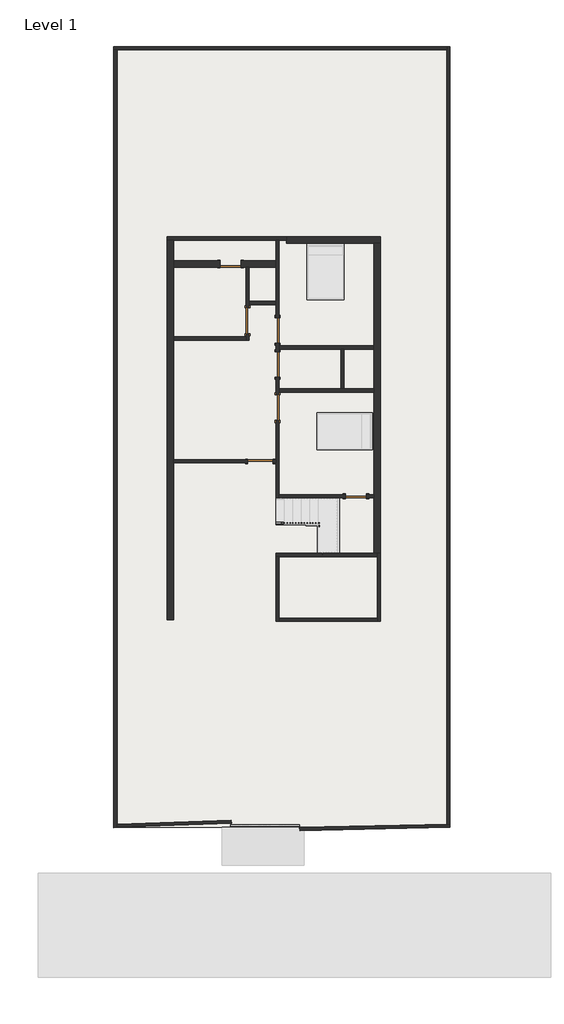
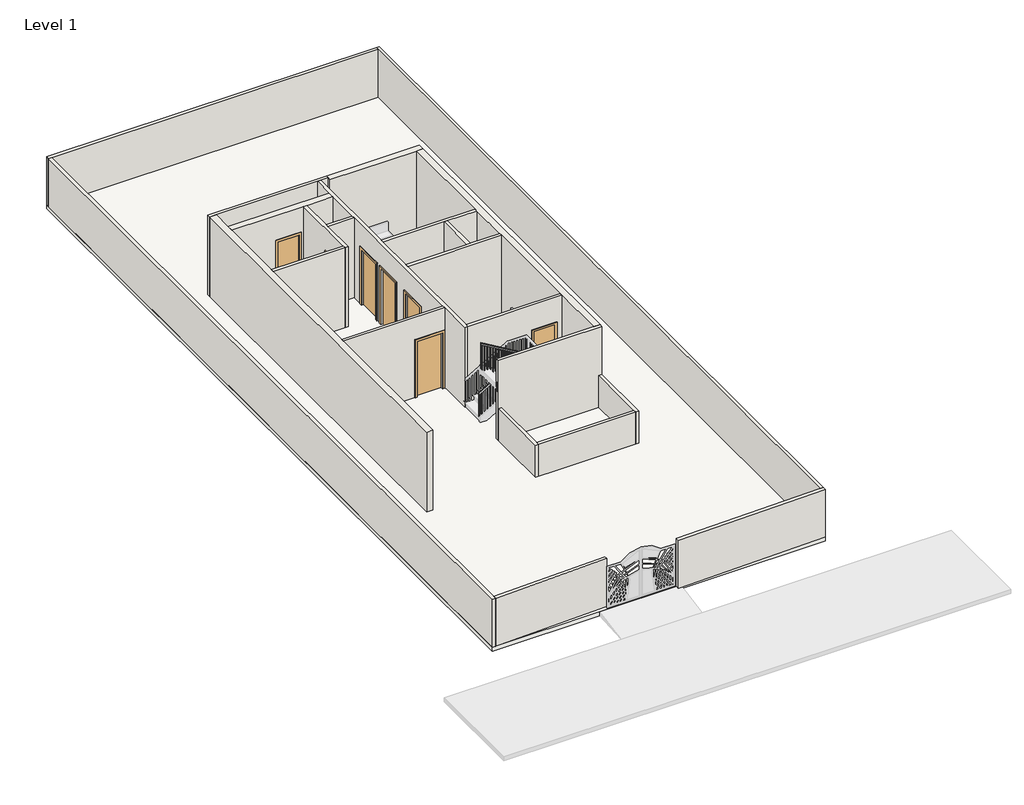
# One storey, part 1 of 2: 23 walls, 7 doors, 1 railing, 1 slab.
"""IFC4 building model written with IfcOpenShell, lengths in millimetres."""

from ifc_helpers import new_model, si_unit, frame, origin, origin_with_axes, place, context, project, spatial, polyline, outline, extrude, faceted_brep, transform, mapped, element, save
from components import door_85036156, door_d8f5dbb5, door_305aa2a5, door_e5f9f3c4

model = new_model("IFC4")

# Units and contexts
model_context = context("Model", 3, world=origin())
ifc_project = project(units=[si_unit("LENGTHUNIT", "METRE", prefix="MILLI")], contexts=[model_context])

# Site, building, storey
site = spatial("IfcSite", under=ifc_project)
building = spatial("IfcBuilding", under=site)
storey = spatial("IfcBuildingStorey", under=building, Name="Level 1", Elevation=0.0)

# Doors
placement = place(None, origin())
door_shape = door_85036156(model_context)
element("IfcDoor", 1, ObjectType="Single-Flush : 30\" x 80\"", at=placement, inside=storey, context=model_context, shape_type="MappedRepresentation", body=[
    mapped(door_shape, transform((-2798.2915084, 6430.9935985, 0.0), x_axis=(1.0, 0.0, 0.0), y_axis=(0.0, 1.0, 0.0), z_axis=(0.0, 0.0, 1.0))),
])
door_2_shape = door_d8f5dbb5(model_context)
element("IfcDoor", 2, ObjectType="Single-Flush : 30\" x 80\"", at=placement, inside=storey, context=model_context, shape_type="MappedRepresentation", body=[
    mapped(door_2_shape, transform((1678.4584916, -1855.7564015, 0.0), x_axis=(-1.0, 0.0, 0.0), y_axis=(0.0, -1.0, 0.0), z_axis=(0.0, 0.0, 1.0))),
])
door_3_shape = door_305aa2a5(model_context)
element("IfcDoor", 3, ObjectType="Single-Flush : 36\" x 84\"", at=placement, inside=storey, context=model_context, shape_type="MappedRepresentation", body=[
    mapped(door_3_shape, transform((-2188.6915084, 4405.3435985, 0.0), x_axis=(0.0, -1.0, 0.0), y_axis=(1.0, 0.0, 0.0), z_axis=(0.0, 0.0, 1.0))),
])
element("IfcDoor", 4, ObjectType="Single-Flush : 36\" x 84\"", at=placement, inside=storey, context=model_context, shape_type="MappedRepresentation", body=[
    mapped(door_3_shape, transform((-1121.8915084, 1306.5435985, 0.0), x_axis=(0.0, 1.0, 0.0), y_axis=(-1.0, 0.0, 0.0), z_axis=(0.0, 0.0, 1.0))),
])
door_4_shape = door_e5f9f3c4(model_context)
element("IfcDoor", 5, ObjectType="Single-Flush : 36\" x 84\"", at=placement, inside=storey, context=model_context, shape_type="MappedRepresentation", body=[
    mapped(door_4_shape, transform((-1121.8915084, 4062.4435985, 0.0), x_axis=(0.0, -1.0, 0.0), y_axis=(1.0, 0.0, 0.0), z_axis=(0.0, 0.0, 1.0))),
])
element("IfcDoor", 6, ObjectType="Single-Flush : 36\" x 84\"", at=placement, inside=storey, context=model_context, shape_type="MappedRepresentation", body=[
    mapped(door_4_shape, transform((-1121.8915084, 2843.2435985, 0.0), x_axis=(0.0, -1.0, 0.0), y_axis=(1.0, 0.0, 0.0), z_axis=(0.0, 0.0, 1.0))),
])
element("IfcDoor", 7, ObjectType="Single-Flush : 36\" x 84\"", at=placement, inside=storey, context=model_context, shape_type="MappedRepresentation", body=[
    mapped(door_4_shape, transform((-1731.4915084, -611.1564015, 0.0), x_axis=(1.0, 0.0, 0.0), y_axis=(0.0, 1.0, 0.0), z_axis=(0.0, 0.0, 1.0))),
])

# Railing
element("IfcRailing", 8, ObjectType="Handrail - Rectangular", at=placement, inside=storey, context=model_context, shape_type="SolidModel", body=[
    faceted_brep([(-1179.0415084, -2776.5064015, 1093.6941176), (-1179.0415084, -2776.5064015, 1034.7569051), (-1179.0415084, -2827.3064015, 1034.7569051), (-1179.0415084, -2827.3064015, 1093.6941176), (268.7584916, -2776.5064015, 1945.3411765), (319.5584916, -2776.5064015, 1916.2863169), (319.5584916, -2827.3064015, 1916.2863169), (268.7584916, -2827.3064015, 1945.3411765), (268.7584916, -2776.5064015, 1990.1647059), (319.5584916, -2776.5064015, 1939.3647059), (319.5584916, -2827.3064015, 1939.3647059), (268.7584916, -2827.3064015, 1990.1647059), (395.7584916, -2776.5064015, 1990.1647059), (395.7584916, -2776.5064015, 1939.3647059), (344.9584916, -2827.3064015, 1939.3647059), (344.9584916, -2827.3064015, 1990.1647059), (395.7584916, -2903.5064015, 1990.1647059), (395.7584916, -2903.5064015, 1939.3647059), (344.9584916, -2903.5064015, 1939.3647059), (344.9584916, -2903.5064015, 1990.1647059), (395.7584916, -2928.9064015, 1990.1647059), (344.9584916, -2928.9064015, 1990.1647059), (344.9584916, -2928.9064015, 1939.3647059), (395.7584916, -2928.9064015, 1939.3647059)], [[[0, 1, 2, 3]], [[1, 0, 4, 5]], [[2, 1, 5, 6]], [[3, 2, 6, 7]], [[0, 3, 7, 4]], [[5, 4, 8, 9]], [[6, 5, 9, 10]], [[7, 6, 10, 11]], [[4, 7, 11, 8]], [[9, 8, 12, 13]], [[10, 9, 13, 14]], [[11, 10, 14, 15]], [[8, 11, 15, 12]], [[13, 12, 16, 17]], [[14, 13, 17, 18]], [[15, 14, 18, 19]], [[12, 15, 19, 16]], [[20, 21, 22, 23]], [[17, 16, 20, 23]], [[18, 17, 23, 22]], [[19, 18, 22, 21]], [[16, 19, 21, 20]]]),
    faceted_brep([(395.7584916, -2903.5064015, 1990.1647059), (395.7584916, -2954.3064015, 1939.3647059), (344.9584916, -2954.3064015, 1939.3647059), (344.9584916, -2903.5064015, 1990.1647059), (395.7584916, -2903.5064015, 2139.5764706), (344.9584916, -2903.5064015, 2110.521611), (344.9584916, -2954.3064015, 2110.521611), (395.7584916, -2954.3064015, 2139.5764706)], [[[0, 1, 2, 3]], [[4, 5, 6, 7]], [[1, 0, 4, 7]], [[2, 1, 7, 6]], [[3, 2, 6, 5]], [[0, 3, 5, 4]]]),
    faceted_brep([(395.7584916, -2954.3064015, 2139.5764706), (344.9584916, -2954.3064015, 2110.521611), (344.9584916, -2903.5064015, 2110.521611), (395.7584916, -2903.5064015, 2139.5764706), (-1179.0415084, -2954.3064015, 3065.9294118), (-1179.0415084, -2903.5064015, 3065.9294118), (-1179.0415084, -2903.5064015, 3006.9921993), (-1179.0415084, -2954.3064015, 3006.9921993)], [[[0, 1, 2, 3]], [[4, 5, 6, 7]], [[1, 0, 4, 7]], [[2, 1, 7, 6]], [[3, 2, 6, 5]], [[0, 3, 5, 4]]]),
    extrude(outline(polyline([(2986.4480816, -1144.1165084), (2997.653964, -1163.1665084), (1972.2352941, -1163.1665084), (1972.2352941, -1144.1165084), (2986.4480816, -1144.1165084)])), frame((0.0, -2938.4314015, 0.0), z_axis=(0.0, 1.0, 0.0), x_axis=(0.0, 0.0, 1.0)), (0.0, 0.0, 1.0), 19.05),
    extrude(outline(polyline([(2926.6833757, -1042.5165084), (2937.8892581, -1061.5665084), (1972.2352941, -1061.5665084), (1972.2352941, -1042.5165084), (2926.6833757, -1042.5165084)])), frame((0.0, -2938.4314015, 0.0), z_axis=(0.0, 1.0, 0.0), x_axis=(0.0, 0.0, 1.0)), (0.0, 0.0, 1.0), 19.05),
    extrude(outline(polyline([(2866.9186699, -940.9165084), (2878.1245522, -959.9665084), (1972.2352941, -959.9665084), (1972.2352941, -940.9165084), (2866.9186699, -940.9165084)])), frame((0.0, -2938.4314015, 0.0), z_axis=(0.0, 1.0, 0.0), x_axis=(0.0, 0.0, 1.0)), (0.0, 0.0, 1.0), 19.05),
    extrude(outline(polyline([(2807.153964, -839.3165084), (2818.3598463, -858.3665084), (1792.9411765, -858.3665084), (1792.9411765, -839.3165084), (2807.153964, -839.3165084)])), frame((0.0, -2938.4314015, 0.0), z_axis=(0.0, 1.0, 0.0), x_axis=(0.0, 0.0, 1.0)), (0.0, 0.0, 1.0), 19.05),
    extrude(outline(polyline([(2747.3892581, -737.7165084), (2758.5951404, -756.7665084), (1792.9411765, -756.7665084), (1792.9411765, -737.7165084), (2747.3892581, -737.7165084)])), frame((0.0, -2938.4314015, 0.0), z_axis=(0.0, 1.0, 0.0), x_axis=(0.0, 0.0, 1.0)), (0.0, 0.0, 1.0), 19.05),
    extrude(outline(polyline([(2687.6245522, -636.1165084), (2698.8304346, -655.1665084), (1792.9411765, -655.1665084), (1792.9411765, -636.1165084), (2687.6245522, -636.1165084)])), frame((0.0, -2938.4314015, 0.0), z_axis=(0.0, 1.0, 0.0), x_axis=(0.0, 0.0, 1.0)), (0.0, 0.0, 1.0), 19.05),
    extrude(outline(polyline([(2627.8598463, -534.5165084), (2639.0657287, -553.5665084), (1613.6470588, -553.5665084), (1613.6470588, -534.5165084), (2627.8598463, -534.5165084)])), frame((0.0, -2938.4314015, 0.0), z_axis=(0.0, 1.0, 0.0), x_axis=(0.0, 0.0, 1.0)), (0.0, 0.0, 1.0), 19.05),
    extrude(outline(polyline([(2568.0951404, -432.9165084), (2579.3010228, -451.9665084), (1613.6470588, -451.9665084), (1613.6470588, -432.9165084), (2568.0951404, -432.9165084)])), frame((0.0, -2938.4314015, 0.0), z_axis=(0.0, 1.0, 0.0), x_axis=(0.0, 0.0, 1.0)), (0.0, 0.0, 1.0), 19.05),
    extrude(outline(polyline([(2508.3304346, -331.3165084), (2519.5363169, -350.3665084), (1613.6470588, -350.3665084), (1613.6470588, -331.3165084), (2508.3304346, -331.3165084)])), frame((0.0, -2938.4314015, 0.0), z_axis=(0.0, 1.0, 0.0), x_axis=(0.0, 0.0, 1.0)), (0.0, 0.0, 1.0), 19.05),
    extrude(outline(polyline([(2448.5657287, -229.7165084), (2459.771611, -248.7665084), (1434.3529412, -248.7665084), (1434.3529412, -229.7165084), (2448.5657287, -229.7165084)])), frame((0.0, -2938.4314015, 0.0), z_axis=(0.0, 1.0, 0.0), x_axis=(0.0, 0.0, 1.0)), (0.0, 0.0, 1.0), 19.05),
    extrude(outline(polyline([(2388.8010228, -128.1165084), (2400.0069051, -147.1665084), (1434.3529412, -147.1665084), (1434.3529412, -128.1165084), (2388.8010228, -128.1165084)])), frame((0.0, -2938.4314015, 0.0), z_axis=(0.0, 1.0, 0.0), x_axis=(0.0, 0.0, 1.0)), (0.0, 0.0, 1.0), 19.05),
    extrude(outline(polyline([(2329.0363169, -26.5165084), (2340.2421993, -45.5665084), (1434.3529412, -45.5665084), (1434.3529412, -26.5165084), (2329.0363169, -26.5165084)])), frame((0.0, -2938.4314015, 0.0), z_axis=(0.0, 1.0, 0.0), x_axis=(0.0, 0.0, 1.0)), (0.0, 0.0, 1.0), 19.05),
    extrude(outline(polyline([(2269.271611, 75.0834916), (2280.4774934, 56.0334916), (1255.0588235, 56.0334916), (1255.0588235, 75.0834916), (2269.271611, 75.0834916)])), frame((0.0, -2938.4314015, 0.0), z_axis=(0.0, 1.0, 0.0), x_axis=(0.0, 0.0, 1.0)), (0.0, 0.0, 1.0), 19.05),
    extrude(outline(polyline([(2209.5069051, 176.6834916), (2220.7127875, 157.6334916), (1255.0588235, 157.6334916), (1255.0588235, 176.6834916), (2209.5069051, 176.6834916)])), frame((0.0, -2938.4314015, 0.0), z_axis=(0.0, 1.0, 0.0), x_axis=(0.0, 0.0, 1.0)), (0.0, 0.0, 1.0), 19.05),
    extrude(outline(polyline([(2149.7421993, 278.2834916), (2160.9480816, 259.2334916), (1255.0588235, 259.2334916), (1255.0588235, 278.2834916), (2149.7421993, 278.2834916)])), frame((0.0, -2938.4314015, 0.0), z_axis=(0.0, 1.0, 0.0), x_axis=(0.0, 0.0, 1.0)), (0.0, 0.0, 1.0), 19.05),
    extrude(outline(polyline([(360.8334916, -2893.9814015), (379.8834916, -2893.9814015), (379.8834916, -2913.0314015), (360.8334916, -2913.0314015), (360.8334916, -2893.9814015)])), frame((0.0, 0.0, 1075.7647059), z_axis=(0.0, 0.0, 1.0), x_axis=(1.0, 0.0, 0.0)), (0.0, 0.0, 1.0), 863.6),
    extrude(outline(polyline([(335.4334916, -2811.4314015), (335.4334916, -2792.3814015), (354.4834916, -2792.3814015), (354.4834916, -2811.4314015), (335.4334916, -2811.4314015)])), frame((0.0, 0.0, 1075.7647059), z_axis=(0.0, 0.0, 1.0), x_axis=(1.0, 0.0, 0.0)), (0.0, 0.0, 1.0), 863.6),
    extrude(outline(polyline([(1877.0657287, 252.8834916), (1865.8598463, 233.8334916), (896.4705882, 233.8334916), (896.4705882, 252.8834916), (1877.0657287, 252.8834916)])), frame((0.0, -2811.4314015, 0.0), z_axis=(0.0, 1.0, 0.0), x_axis=(0.0, 0.0, 1.0)), (0.0, 0.0, 1.0), 19.05),
    extrude(outline(polyline([(1817.3010228, 151.2834916), (1806.0951404, 132.2334916), (896.4705882, 132.2334916), (896.4705882, 151.2834916), (1817.3010228, 151.2834916)])), frame((0.0, -2811.4314015, 0.0), z_axis=(0.0, 1.0, 0.0), x_axis=(0.0, 0.0, 1.0)), (0.0, 0.0, 1.0), 19.05),
    extrude(outline(polyline([(1757.5363169, 49.6834916), (1746.3304346, 30.6334916), (896.4705882, 30.6334916), (896.4705882, 49.6834916), (1757.5363169, 49.6834916)])), frame((0.0, -2811.4314015, 0.0), z_axis=(0.0, 1.0, 0.0), x_axis=(0.0, 0.0, 1.0)), (0.0, 0.0, 1.0), 19.05),
    extrude(outline(polyline([(1697.771611, -51.9165084), (1686.5657287, -70.9665084), (717.1764706, -70.9665084), (717.1764706, -51.9165084), (1697.771611, -51.9165084)])), frame((0.0, -2811.4314015, 0.0), z_axis=(0.0, 1.0, 0.0), x_axis=(0.0, 0.0, 1.0)), (0.0, 0.0, 1.0), 19.05),
    extrude(outline(polyline([(1638.0069051, -153.5165084), (1626.8010228, -172.5665084), (717.1764706, -172.5665084), (717.1764706, -153.5165084), (1638.0069051, -153.5165084)])), frame((0.0, -2811.4314015, 0.0), z_axis=(0.0, 1.0, 0.0), x_axis=(0.0, 0.0, 1.0)), (0.0, 0.0, 1.0), 19.05),
    extrude(outline(polyline([(1578.2421993, -255.1165084), (1567.0363169, -274.1665084), (717.1764706, -274.1665084), (717.1764706, -255.1165084), (1578.2421993, -255.1165084)])), frame((0.0, -2811.4314015, 0.0), z_axis=(0.0, 1.0, 0.0), x_axis=(0.0, 0.0, 1.0)), (0.0, 0.0, 1.0), 19.05),
    extrude(outline(polyline([(1518.4774934, -356.7165084), (1507.271611, -375.7665084), (537.8823529, -375.7665084), (537.8823529, -356.7165084), (1518.4774934, -356.7165084)])), frame((0.0, -2811.4314015, 0.0), z_axis=(0.0, 1.0, 0.0), x_axis=(0.0, 0.0, 1.0)), (0.0, 0.0, 1.0), 19.05),
    extrude(outline(polyline([(1458.7127875, -458.3165084), (1447.5069051, -477.3665084), (537.8823529, -477.3665084), (537.8823529, -458.3165084), (1458.7127875, -458.3165084)])), frame((0.0, -2811.4314015, 0.0), z_axis=(0.0, 1.0, 0.0), x_axis=(0.0, 0.0, 1.0)), (0.0, 0.0, 1.0), 19.05),
    extrude(outline(polyline([(1398.9480816, -559.9165084), (1387.7421993, -578.9665084), (537.8823529, -578.9665084), (537.8823529, -559.9165084), (1398.9480816, -559.9165084)])), frame((0.0, -2811.4314015, 0.0), z_axis=(0.0, 1.0, 0.0), x_axis=(0.0, 0.0, 1.0)), (0.0, 0.0, 1.0), 19.05),
    extrude(outline(polyline([(1339.1833757, -661.5165084), (1327.9774934, -680.5665084), (358.5882353, -680.5665084), (358.5882353, -661.5165084), (1339.1833757, -661.5165084)])), frame((0.0, -2811.4314015, 0.0), z_axis=(0.0, 1.0, 0.0), x_axis=(0.0, 0.0, 1.0)), (0.0, 0.0, 1.0), 19.05),
    extrude(outline(polyline([(1279.4186699, -763.1165084), (1268.2127875, -782.1665084), (358.5882353, -782.1665084), (358.5882353, -763.1165084), (1279.4186699, -763.1165084)])), frame((0.0, -2811.4314015, 0.0), z_axis=(0.0, 1.0, 0.0), x_axis=(0.0, 0.0, 1.0)), (0.0, 0.0, 1.0), 19.05),
    extrude(outline(polyline([(1219.653964, -864.7165084), (1208.4480816, -883.7665084), (358.5882353, -883.7665084), (358.5882353, -864.7165084), (1219.653964, -864.7165084)])), frame((0.0, -2811.4314015, 0.0), z_axis=(0.0, 1.0, 0.0), x_axis=(0.0, 0.0, 1.0)), (0.0, 0.0, 1.0), 19.05),
    extrude(outline(polyline([(1159.8892581, -966.3165084), (1148.6833757, -985.3665084), (179.2941176, -985.3665084), (179.2941176, -966.3165084), (1159.8892581, -966.3165084)])), frame((0.0, -2811.4314015, 0.0), z_axis=(0.0, 1.0, 0.0), x_axis=(0.0, 0.0, 1.0)), (0.0, 0.0, 1.0), 19.05),
    extrude(outline(polyline([(1100.1245522, -1067.9165084), (1088.9186699, -1086.9665084), (179.2941176, -1086.9665084), (179.2941176, -1067.9165084), (1100.1245522, -1067.9165084)])), frame((0.0, -2811.4314015, 0.0), z_axis=(0.0, 1.0, 0.0), x_axis=(0.0, 0.0, 1.0)), (0.0, 0.0, 1.0), 19.05),
    extrude(outline(polyline([(360.8334916, -2919.3814015), (379.8834916, -2919.3814015), (379.8834916, -2938.4314015), (360.8334916, -2938.4314015), (360.8334916, -2919.3814015)])), frame((0.0, 0.0, 1075.7647059), z_axis=(0.0, 0.0, 1.0), x_axis=(1.0, 0.0, 0.0)), (0.0, 0.0, 1.0), 863.6),
    extrude(outline(polyline([(360.8334916, -2811.4314015), (360.8334916, -2792.3814015), (379.8834916, -2792.3814015), (379.8834916, -2811.4314015), (360.8334916, -2811.4314015)])), frame((0.0, 0.0, 1075.7647059), z_axis=(0.0, 0.0, 1.0), x_axis=(1.0, 0.0, 0.0)), (0.0, 0.0, 1.0), 863.6),
    extrude(outline(polyline([(2995.7863169, -1159.9915084), (3006.9921993, -1179.0415084), (1972.2352941, -1179.0415084), (1972.2352941, -1159.9915084), (2995.7863169, -1159.9915084)])), frame((0.0, -2938.4314015, 0.0), z_axis=(0.0, 1.0, 0.0), x_axis=(0.0, 0.0, 1.0)), (0.0, 0.0, 1.0), 19.05),
    extrude(outline(polyline([(1045.9627875, -1159.9915084), (1034.7569051, -1179.0415084), (179.2941176, -1179.0415084), (179.2941176, -1159.9915084), (1045.9627875, -1159.9915084)])), frame((0.0, -2811.4314015, 0.0), z_axis=(0.0, 1.0, 0.0), x_axis=(0.0, 0.0, 1.0)), (0.0, 0.0, 1.0), 19.05),
])

# Slab
element("IfcSlab", 9, ObjectType="Generic - 12\"", at=placement, inside=storey, context=model_context, shape_type="SweptSolid", body=[
    extrude(outline(polyline([(5035.3021219, 14183.4869538), (5035.3021219, -13665.8789629), (-6966.1978781, -13665.8789629), (-6966.1978781, 14183.4869538), (5035.3021219, 14183.4869538)])), frame((0.0, 0.0, -152.4), z_axis=(0.0, 0.0, 1.0), x_axis=(1.0, 0.0, 0.0)), (0.0, 0.0, 1.0), 152.4),
])

# Walls
element("IfcWall", 10, ObjectType="WALL 9\"", at=placement, inside=storey, context=model_context, shape_type="Brep", body=[
    faceted_brep([(-798.0415084, 7167.5935985, 0.0), (2326.1584916, 7167.5935985, 0.0), (2554.7584916, 7167.5935985, 0.0), (2554.7584916, 7167.5935985, 3048.0), (2326.1584916, 7167.5935985, 3048.0), (-798.0415084, 7167.5935985, 3048.0), (-798.0415084, 7396.1935985, 0.0), (-798.0415084, 7396.1935985, 3048.0), (2554.7584916, 7396.1935985, 3048.0), (2554.7584916, 7396.1935985, 0.0), (-798.0415084, 7281.8935985, 0.0), (-798.0415084, 7281.8935985, 3048.0)], [[[0, 1, 2, 3, 4, 5]], [[6, 7, 8, 9]], [[2, 1, 0, 10, 6, 9]], [[0, 5, 11, 7, 6, 10]], [[3, 2, 9, 8]], [[5, 4, 3, 8, 7, 11]]]),
])
element("IfcWall", 11, ObjectType="WALL 9\"", at=placement, inside=storey, context=model_context, shape_type="Brep", body=[
    faceted_brep([(2326.1584916, 7167.5935985, 0.0), (2326.1584916, 3509.9935985, 0.0), (2326.1584916, 3395.6935985, 0.0), (2326.1584916, 1973.2935985, 0.0), (2326.1584916, 1858.9935985, 0.0), (2326.1584916, -1798.6064015, 0.0), (2326.1584916, -1912.9064015, 0.0), (2326.1584916, -3894.1064015, 0.0), (2326.1584916, -3894.1064015, 3048.0), (2326.1584916, -1912.9064015, 3048.0), (2326.1584916, -1798.6064015, 3048.0), (2326.1584916, 1858.9935985, 3048.0), (2326.1584916, 1973.2935985, 3048.0), (2326.1584916, 3395.6935985, 3048.0), (2326.1584916, 3509.9935985, 3048.0), (2326.1584916, 7167.5935985, 3048.0), (2554.7584916, 7167.5935985, 0.0), (2554.7584916, 7167.5935985, 3048.0), (2554.7584916, -3894.1064015, 3048.0), (2554.7584916, -3894.1064015, 1219.2), (2554.7584916, -3894.1064015, 0.0), (2440.4584916, -3894.1064015, 0.0)], [[[0, 1, 2, 3, 4, 5, 6, 7, 8, 9, 10, 11, 12, 13, 14, 15]], [[16, 17, 18, 19, 20]], [[7, 6, 5, 4, 3, 2, 1, 0, 16, 20, 21]], [[0, 15, 17, 16]], [[8, 7, 21, 20, 19, 18]], [[15, 14, 13, 12, 11, 10, 9, 8, 18, 17]]]),
])
element("IfcWall", 12, ObjectType="WALL 9\"", at=placement, inside=storey, context=model_context, shape_type="Brep", body=[
    faceted_brep([(-5065.2415084, 7281.8935985, 0.0), (-5065.2415084, -6262.6564015, 0.0), (-5065.2415084, -6262.6564015, 3048.0), (-5065.2415084, 7281.8935985, 3048.0), (-4836.6415084, 7281.8935985, 0.0), (-4836.6415084, 7281.8935985, 3048.0), (-4836.6415084, 6545.2935985, 3048.0), (-4836.6415084, 6316.6935985, 3048.0), (-4836.6415084, 3827.4935985, 3048.0), (-4836.6415084, 3713.1935985, 3048.0), (-4836.6415084, -554.0064015, 3048.0), (-4836.6415084, -668.3064015, 3048.0), (-4836.6415084, -6262.6564015, 3048.0), (-4836.6415084, -6262.6564015, 0.0), (-4836.6415084, -668.3064015, 0.0), (-4836.6415084, -554.0064015, 0.0), (-4836.6415084, 3713.1935985, 0.0), (-4836.6415084, 3827.4935985, 0.0), (-4836.6415084, 6316.6935985, 0.0), (-4836.6415084, 6545.2935985, 0.0)], [[[0, 1, 2, 3]], [[4, 5, 6, 7, 8, 9, 10, 11, 12, 13, 14, 15, 16, 17, 18, 19]], [[1, 0, 4, 19, 18, 17, 16, 15, 14, 13]], [[2, 1, 13, 12]], [[0, 3, 5, 4]], [[3, 2, 12, 11, 10, 9, 8, 7, 6, 5]]]),
])
element("IfcWall", 13, ObjectType="WALL 9\"", at=placement, inside=storey, context=model_context, shape_type="Brep", body=[
    faceted_brep([(-2417.2915084, 6316.6935985, 2032.0), (-2417.2915084, 6316.6935985, 0.0), (-2245.8415084, 6316.6935985, 0.0), (-2131.5415084, 6316.6935985, 0.0), (-1179.0415084, 6316.6935985, 0.0), (-1179.0415084, 6316.6935985, 3048.0), (-2131.5415084, 6316.6935985, 3048.0), (-2245.8415084, 6316.6935985, 3048.0), (-4836.6415084, 6316.6935985, 3048.0), (-4836.6415084, 6316.6935985, 0.0), (-3179.2915084, 6316.6935985, 0.0), (-3179.2915084, 6316.6935985, 2032.0), (-1179.0415084, 6545.2935985, 0.0), (-2417.2915084, 6545.2935985, 0.0), (-2417.2915084, 6545.2935985, 2032.0), (-3179.2915084, 6545.2935985, 2032.0), (-3179.2915084, 6545.2935985, 0.0), (-4836.6415084, 6545.2935985, 0.0), (-4836.6415084, 6545.2935985, 3048.0), (-1179.0415084, 6545.2935985, 3048.0)], [[[0, 1, 2, 3, 4, 5, 6, 7, 8, 9, 10, 11]], [[12, 13, 14, 15, 16, 17, 18, 19]], [[10, 9, 17, 16]], [[4, 3, 2, 1, 13, 12]], [[9, 8, 18, 17]], [[5, 4, 12, 19]], [[14, 13, 1, 0]], [[15, 14, 0, 11]], [[16, 15, 11, 10]], [[8, 7, 6, 5, 19, 18]]]),
])
element("IfcWall", 14, ObjectType="WALL4.5\"", at=placement, inside=storey, context=model_context, shape_type="Brep", body=[
    faceted_brep([(-5065.2415084, 7281.8935985, 0.0), (-4836.6415084, 7281.8935985, 0.0), (-1179.0415084, 7281.8935985, 0.0), (-1064.7415084, 7281.8935985, 0.0), (-798.0415084, 7281.8935985, 0.0), (-798.0415084, 7281.8935985, 3048.0), (-1064.7415084, 7281.8935985, 3048.0), (-1179.0415084, 7281.8935985, 3048.0), (-4836.6415084, 7281.8935985, 3048.0), (-5065.2415084, 7281.8935985, 3048.0), (-5065.2415084, 7396.1935985, 0.0), (-5065.2415084, 7396.1935985, 3048.0), (-798.0415084, 7396.1935985, 3048.0), (-798.0415084, 7396.1935985, 0.0)], [[[0, 1, 2, 3, 4, 5, 6, 7, 8, 9]], [[10, 11, 12, 13]], [[4, 3, 2, 1, 0, 10, 13]], [[5, 4, 13, 12]], [[0, 9, 11, 10]], [[9, 8, 7, 6, 5, 12, 11]]]),
])
element("IfcWall", 15, ObjectType="WALL4.5\"", at=placement, inside=storey, context=model_context, shape_type="Brep", body=[
    faceted_brep([(2554.7584916, -6319.8064015, 0.0), (2554.7584916, -3894.1064015, 0.0), (2554.7584916, -3894.1064015, 1219.2), (2554.7584916, -4008.4064015, 1219.2), (2554.7584916, -6319.8064015, 1219.2), (2440.4584916, -6319.8064015, 0.0), (2440.4584916, -6319.8064015, 1219.2), (2440.4584916, -6205.5064015, 1219.2), (2440.4584916, -4008.4064015, 1219.2), (2440.4584916, -3894.1064015, 1219.2), (2440.4584916, -3894.1064015, 0.0), (2440.4584916, -4008.4064015, 0.0), (2440.4584916, -6205.5064015, 0.0)], [[[0, 1, 2, 3, 4]], [[5, 6, 7, 8, 9, 10, 11, 12]], [[1, 0, 5, 12, 11, 10]], [[4, 3, 2, 9, 8, 7, 6]], [[2, 1, 10, 9]], [[0, 4, 6, 5]]]),
])
element("IfcWall", 16, ObjectType="WALL4.5\"", at=placement, inside=storey, context=model_context, shape_type="Brep", body=[
    faceted_brep([(2440.4584916, -3894.1064015, 0.0), (2326.1584916, -3894.1064015, 0.0), (-1179.0415084, -3894.1064015, 0.0), (-1179.0415084, -3894.1064015, 3048.0), (2326.1584916, -3894.1064015, 3048.0), (2554.7584916, -3894.1064015, 3048.0), (2554.7584916, -3894.1064015, 1219.2), (2440.4584916, -3894.1064015, 1219.2), (2440.4584916, -4008.4064015, 0.0), (2440.4584916, -4008.4064015, 1219.2), (2554.7584916, -4008.4064015, 1219.2), (2554.7584916, -4008.4064015, 3048.0), (-1179.0415084, -4008.4064015, 3048.0), (-1179.0415084, -4008.4064015, 1219.2), (-1179.0415084, -4008.4064015, 0.0), (-1064.7415084, -4008.4064015, 0.0)], [[[0, 1, 2, 3, 4, 5, 6, 7]], [[8, 9, 10, 11, 12, 13, 14, 15]], [[2, 1, 0, 8, 15, 14]], [[3, 2, 14, 13, 12]], [[6, 10, 9, 7]], [[0, 7, 9, 8]], [[6, 5, 11, 10]], [[5, 4, 3, 12, 11]]]),
])
element("IfcWall", 17, ObjectType="WALL4.5\"", at=placement, inside=storey, context=model_context, shape_type="Brep", body=[
    faceted_brep([(-2245.8415084, 3948.1435985, 2133.6), (-2245.8415084, 3948.1435985, 0.0), (-2245.8415084, 3827.4935985, 0.0), (-2245.8415084, 3713.1935985, 0.0), (-2245.8415084, 3713.1935985, 3048.0), (-2245.8415084, 3827.4935985, 3048.0), (-2245.8415084, 6316.6935985, 3048.0), (-2245.8415084, 6316.6935985, 0.0), (-2245.8415084, 4862.5435985, 0.0), (-2245.8415084, 4862.5435985, 2133.6), (-2131.5415084, 3713.1935985, 0.0), (-2131.5415084, 3948.1435985, 0.0), (-2131.5415084, 3948.1435985, 2133.6), (-2131.5415084, 4862.5435985, 2133.6), (-2131.5415084, 4862.5435985, 0.0), (-2131.5415084, 4983.1935985, 0.0), (-2131.5415084, 5097.4935985, 0.0), (-2131.5415084, 6316.6935985, 0.0), (-2131.5415084, 6316.6935985, 3048.0), (-2131.5415084, 5097.4935985, 3048.0), (-2131.5415084, 4983.1935985, 3048.0), (-2131.5415084, 3713.1935985, 3048.0)], [[[0, 1, 2, 3, 4, 5, 6, 7, 8, 9]], [[10, 11, 12, 13, 14, 15, 16, 17, 18, 19, 20, 21]], [[8, 7, 17, 16, 15, 14]], [[3, 2, 1, 11, 10]], [[7, 6, 18, 17]], [[4, 3, 10, 21]], [[12, 11, 1, 0]], [[13, 12, 0, 9]], [[14, 13, 9, 8]], [[6, 5, 4, 21, 20, 19, 18]]]),
])
element("IfcWall", 18, ObjectType="WALL4.5\"", at=placement, inside=storey, context=model_context, shape_type="SweptSolid", body=[
    extrude(outline(polyline([(-2245.8415084, 3713.1935985), (-4836.6415084, 3713.1935985), (-4836.6415084, 3827.4935985), (-2245.8415084, 3827.4935985), (-2245.8415084, 3713.1935985)])), origin_with_axes(), (0.0, 0.0, 1.0), 3048.0),
])
element("IfcWall", 19, ObjectType="WALL4.5\"", at=placement, inside=storey, context=model_context, shape_type="SweptSolid", body=[
    extrude(outline(polyline([(-1179.0415084, 4983.1935985), (-2131.5415084, 4983.1935985), (-2131.5415084, 5097.4935985), (-1179.0415084, 5097.4935985), (-1179.0415084, 4983.1935985)])), origin_with_axes(), (0.0, 0.0, 1.0), 3048.0),
])
element("IfcWall", 20, ObjectType="WALL4.5\"", at=placement, inside=storey, context=model_context, shape_type="Brep", body=[
    faceted_brep([(-1179.0415084, 2386.0435985, 0.0), (-1179.0415084, 1763.7435985, 0.0), (-1179.0415084, 1763.7435985, 2133.6), (-1179.0415084, 849.3435985, 2133.6), (-1179.0415084, 849.3435985, 0.0), (-1179.0415084, -554.0064015, 0.0), (-1179.0415084, -668.3064015, 0.0), (-1179.0415084, -1912.9064015, 0.0), (-1179.0415084, -1912.9064015, 3048.0), (-1179.0415084, -668.3064015, 3048.0), (-1179.0415084, -554.0064015, 3048.0), (-1179.0415084, 4983.1935985, 3048.0), (-1179.0415084, 5097.4935985, 3048.0), (-1179.0415084, 6316.6935985, 3048.0), (-1179.0415084, 6545.2935985, 3048.0), (-1179.0415084, 7281.8935985, 3048.0), (-1179.0415084, 7281.8935985, 0.0), (-1179.0415084, 6545.2935985, 0.0), (-1179.0415084, 6316.6935985, 0.0), (-1179.0415084, 5097.4935985, 0.0), (-1179.0415084, 4983.1935985, 0.0), (-1179.0415084, 4519.6435985, 0.0), (-1179.0415084, 4519.6435985, 2133.6), (-1179.0415084, 3605.2435985, 2133.6), (-1179.0415084, 3605.2435985, 0.0), (-1179.0415084, 3300.4435985, 0.0), (-1179.0415084, 3300.4435985, 2133.6), (-1179.0415084, 2386.0435985, 2133.6), (-1064.7415084, 1763.7435985, 2133.6), (-1064.7415084, 1763.7435985, 0.0), (-1064.7415084, 1858.9935985, 0.0), (-1064.7415084, 1973.2935985, 0.0), (-1064.7415084, 2386.0435985, 0.0), (-1064.7415084, 2386.0435985, 2133.6), (-1064.7415084, 3300.4435985, 2133.6), (-1064.7415084, 3300.4435985, 0.0), (-1064.7415084, 3395.6935985, 0.0), (-1064.7415084, 3509.9935985, 0.0), (-1064.7415084, 3605.2435985, 0.0), (-1064.7415084, 3605.2435985, 2133.6), (-1064.7415084, 4519.6435985, 2133.6), (-1064.7415084, 4519.6435985, 0.0), (-1064.7415084, 7281.8935985, 0.0), (-1064.7415084, 7281.8935985, 3048.0), (-1064.7415084, 3509.9935985, 3048.0), (-1064.7415084, 3395.6935985, 3048.0), (-1064.7415084, 1973.2935985, 3048.0), (-1064.7415084, 1858.9935985, 3048.0), (-1064.7415084, -1798.6064015, 3048.0), (-1064.7415084, -1912.9064015, 3048.0), (-1064.7415084, -1912.9064015, 0.0), (-1064.7415084, -1798.6064015, 0.0), (-1064.7415084, 849.3435985, 0.0), (-1064.7415084, 849.3435985, 2133.6)], [[[0, 1, 2, 3, 4, 5, 6, 7, 8, 9, 10, 11, 12, 13, 14, 15, 16, 17, 18, 19, 20, 21, 22, 23, 24, 25, 26, 27]], [[28, 29, 30, 31, 32, 33, 34, 35, 36, 37, 38, 39, 40, 41, 42, 43, 44, 45, 46, 47, 48, 49, 50, 51, 52, 53]], [[21, 20, 19, 18, 17, 16, 42, 41]], [[25, 24, 38, 37, 36, 35]], [[52, 51, 50, 7, 6, 5, 4]], [[32, 31, 30, 29, 1, 0]], [[16, 15, 43, 42]], [[8, 7, 50, 49]], [[39, 38, 24, 23]], [[40, 39, 23, 22]], [[41, 40, 22, 21]], [[33, 32, 0, 27]], [[34, 33, 27, 26]], [[35, 34, 26, 25]], [[2, 1, 29, 28]], [[3, 2, 28, 53]], [[4, 3, 53, 52]], [[15, 14, 13, 12, 11, 10, 9, 8, 49, 48, 47, 46, 45, 44, 43]]]),
])
element("IfcWall", 21, ObjectType="WALL4.5\"", at=placement, inside=storey, context=model_context, shape_type="SweptSolid", body=[
    extrude(outline(polyline([(0.0, -1064.7415084), (0.0, 1297.4584916), (2032.0, 1297.4584916), (2032.0, 2059.4584916), (0.0, 2059.4584916), (0.0, 2326.1584916), (3048.0, 2326.1584916), (3048.0, -1064.7415084), (0.0, -1064.7415084)])), frame((0.0, -1912.9064015, 0.0), z_axis=(0.0, 1.0, 0.0), x_axis=(0.0, 0.0, 1.0)), (0.0, 0.0, 1.0), 114.3),
])
element("IfcWall", 22, ObjectType="WALL4.5\"", at=placement, inside=storey, context=model_context, shape_type="Brep", body=[
    faceted_brep([(-1064.7415084, 3395.6935985, 0.0), (1145.0584916, 3395.6935985, 0.0), (1259.3584916, 3395.6935985, 0.0), (2326.1584916, 3395.6935985, 0.0), (2326.1584916, 3395.6935985, 3048.0), (1259.3584916, 3395.6935985, 3048.0), (1145.0584916, 3395.6935985, 3048.0), (-1064.7415084, 3395.6935985, 3048.0), (-1064.7415084, 3509.9935985, 0.0), (-1064.7415084, 3509.9935985, 3048.0), (2326.1584916, 3509.9935985, 3048.0), (2326.1584916, 3509.9935985, 0.0)], [[[0, 1, 2, 3, 4, 5, 6, 7]], [[8, 9, 10, 11]], [[3, 2, 1, 0, 8, 11]], [[4, 3, 11, 10]], [[0, 7, 9, 8]], [[7, 6, 5, 4, 10, 9]]]),
])
element("IfcWall", 23, ObjectType="WALL4.5\"", at=placement, inside=storey, context=model_context, shape_type="SweptSolid", body=[
    extrude(outline(polyline([(1259.3584916, 3395.6935985), (1259.3584916, 1973.2935985), (1145.0584916, 1973.2935985), (1145.0584916, 3395.6935985), (1259.3584916, 3395.6935985)])), origin_with_axes(), (0.0, 0.0, 1.0), 3048.0),
])
element("IfcWall", 24, ObjectType="WALL4.5\"", at=placement, inside=storey, context=model_context, shape_type="Brep", body=[
    faceted_brep([(-1064.7415084, 1858.9935985, 0.0), (2326.1584916, 1858.9935985, 0.0), (2326.1584916, 1858.9935985, 3048.0), (-1064.7415084, 1858.9935985, 3048.0), (-1064.7415084, 1973.2935985, 0.0), (-1064.7415084, 1973.2935985, 3048.0), (1145.0584916, 1973.2935985, 3048.0), (1259.3584916, 1973.2935985, 3048.0), (2326.1584916, 1973.2935985, 3048.0), (2326.1584916, 1973.2935985, 0.0), (1259.3584916, 1973.2935985, 0.0), (1145.0584916, 1973.2935985, 0.0)], [[[0, 1, 2, 3]], [[4, 5, 6, 7, 8, 9, 10, 11]], [[1, 0, 4, 11, 10, 9]], [[2, 1, 9, 8]], [[0, 3, 5, 4]], [[3, 2, 8, 7, 6, 5]]]),
])
element("IfcWall", 25, ObjectType="WALL4.5\"", at=placement, inside=storey, context=model_context, shape_type="SweptSolid", body=[
    extrude(outline(polyline([(2133.6, -1274.2915084), (0.0, -1274.2915084), (0.0, -1179.0415084), (3048.0, -1179.0415084), (3048.0, -4836.6415084), (0.0, -4836.6415084), (0.0, -2188.6915084), (2133.6, -2188.6915084), (2133.6, -1274.2915084)])), frame((0.0, -668.3064015, 0.0), z_axis=(0.0, 1.0, 0.0), x_axis=(0.0, 0.0, 1.0)), (0.0, 0.0, 1.0), 114.3),
])
element("IfcWall", 26, ObjectType="WALL4.5\"", at=placement, inside=storey, context=model_context, shape_type="Brep", body=[
    faceted_brep([(-1179.0415084, -4008.4064015, 0.0), (-1179.0415084, -6319.8064015, 0.0), (-1179.0415084, -6319.8064015, 1219.2), (-1179.0415084, -4008.4064015, 1219.2), (-1064.7415084, -4008.4064015, 0.0), (-1064.7415084, -4008.4064015, 1219.2), (-1064.7415084, -6205.5064015, 1219.2), (-1064.7415084, -6319.8064015, 1219.2), (-1064.7415084, -6319.8064015, 0.0), (-1064.7415084, -6205.5064015, 0.0)], [[[0, 1, 2, 3]], [[4, 5, 6, 7, 8, 9]], [[1, 0, 4, 9, 8]], [[3, 2, 7, 6, 5]], [[0, 3, 5, 4]], [[2, 1, 8, 7]]]),
])
element("IfcWall", 27, ObjectType="WALL4.5\"", at=placement, inside=storey, context=model_context, shape_type="Brep", body=[
    faceted_brep([(-6966.1978781, 14069.1869538, 0.0), (-6851.8978781, 14069.1869538, 0.0), (4921.0021219, 14069.1869538, 0.0), (4921.0021219, 14069.1869538, 1828.8), (-6851.8978781, 14069.1869538, 1828.8), (-6966.1978781, 14069.1869538, 1828.8), (-6966.1978781, 14183.4869538, 0.0), (-6966.1978781, 14183.4869538, 1828.8), (4921.0021219, 14183.4869538, 1828.8), (4921.0021219, 14183.4869538, 0.0)], [[[0, 1, 2, 3, 4, 5]], [[6, 7, 8, 9]], [[2, 1, 0, 6, 9]], [[5, 4, 3, 8, 7]], [[0, 5, 7, 6]], [[3, 2, 9, 8]]]),
])
element("IfcWall", 28, ObjectType="WALL4.5\"", at=placement, inside=storey, context=model_context, shape_type="Brep", body=[
    faceted_brep([(-6851.8978781, -13665.6869951, 0.0), (-6851.8978781, -13551.3173242, 0.0), (-6851.8978781, 14069.1869538, 0.0), (-6851.8978781, 14069.1869538, 1828.8), (-6851.8978781, -13551.3173242, 1828.8), (-6851.8978781, -13665.6869951, 1828.8), (-6966.1978781, -13669.6784391, 0.0), (-6966.1978781, -13669.6784391, 1828.8), (-6966.1978781, 14069.1869538, 1828.8), (-6966.1978781, 14069.1869538, 0.0)], [[[0, 1, 2, 3, 4, 5]], [[6, 7, 8, 9]], [[2, 1, 0, 6, 9]], [[5, 4, 3, 8, 7]], [[0, 5, 7, 6]], [[3, 2, 9, 8]]]),
])
element("IfcWall", 29, ObjectType="WALL4.5\"", at=placement, inside=storey, context=model_context, shape_type="Brep", body=[
    faceted_brep([(5035.3021219, -13552.0823715, 0.0), (4921.0021219, -13554.5437209, 0.0), (-329.7046313, -13667.6130462, 0.0), (-329.7046313, -13667.6130462, 1828.8), (4921.0021219, -13554.5437209, 1828.8), (5035.3021219, -13552.0823715, 1828.8), (5035.3021219, -13666.4088699, 0.0), (5035.3021219, -13666.4088699, 1828.8), (-327.2438524, -13781.8865539, 1828.8), (-327.2438524, -13781.8865539, 0.0)], [[[0, 1, 2, 3, 4, 5]], [[6, 7, 8, 9]], [[2, 1, 0, 6, 9]], [[3, 2, 9, 8]], [[5, 4, 3, 8, 7]], [[0, 5, 7, 6]]]),
])
element("IfcWall", 30, ObjectType="WALL4.5\"", at=placement, inside=storey, context=model_context, shape_type="Brep", body=[
    faceted_brep([(4921.0021219, 14183.4869538, 0.0), (4921.0021219, 14069.1869538, 0.0), (4921.0021219, -13554.5437209, 0.0), (4921.0021219, -13554.5437209, 1828.8), (4921.0021219, 14069.1869538, 1828.8), (4921.0021219, 14183.4869538, 1828.8), (5035.3021219, 14183.4869538, 0.0), (5035.3021219, 14183.4869538, 1828.8), (5035.3021219, -13552.0823715, 1828.8), (5035.3021219, -13552.0823715, 0.0)], [[[0, 1, 2, 3, 4, 5]], [[6, 7, 8, 9]], [[2, 1, 0, 6, 9]], [[5, 4, 3, 8, 7]], [[0, 5, 7, 6]], [[3, 2, 9, 8]]]),
])
element("IfcWall", 31, ObjectType="WALL4.5\"", at=placement, inside=storey, context=model_context, shape_type="SweptSolid", body=[
    extrude(outline(polyline([(2440.4584916, -6319.8064015), (-1064.7415084, -6319.8064015), (-1064.7415084, -6205.5064015), (2440.4584916, -6205.5064015), (2440.4584916, -6319.8064015)])), origin_with_axes(), (0.0, 0.0, 1.0), 1219.2),
])
element("IfcWall", 32, ObjectType="WALL4.5\"", at=placement, inside=storey, context=model_context, shape_type="SweptSolid", body=[
    extrude(outline(polyline([(-6851.8978781, -13551.3173242), (-2771.369976, -13408.8221499), (-2767.3809636, -13523.0525215), (-6851.8978781, -13665.6869951), (-6851.8978781, -13551.3173242)])), origin_with_axes(), (0.0, 0.0, 1.0), 1828.8),
])

save(model, "model.ifc")

# Revit data of these elements
# Type "Single-Flush : 30\" x 80\""
#   Type Mark = "5"
#   Construction Type Id = "MDOOR"
#   Assembly Code = "C1020"
#   Analytic Construction = "Metal"
#   Thickness = 0' - 2"
#   Heat Transfer Coefficient (U) = 0.651978 BTU/(h·ft²·°F)
#   Height = 6' - 8"
#   Trim Projection Ext = 0' - 1"
#   Trim Projection Int = 0' - 1"
#   Trim Width = 0' - 3"
#   Width = 2' - 6"
#   Define Thermal Properties by = 1
#   Define Thermal Properties by = 1
#   Door Material = Door - Panel
#   Frame Material = Door - Frame
#   Visual Light Transmittance = 0
#   Solar Heat Gain Coefficient = 0
#   Function = (empty or 0)
#   Wall Closure = (empty or 0)
# Type "Single-Flush : 36\" x 84\""
#   Type Mark = "1"
#   Construction Type Id = "MDOOR"
#   Assembly Code = "C1020"
#   Analytic Construction = "Metal"
#   Thickness = 0' - 2"
#   Heat Transfer Coefficient (U) = 0.651978 BTU/(h·ft²·°F)
#   Height = 7' - 0"
#   Trim Projection Ext = 0' - 1"
#   Trim Projection Int = 0' - 1"
#   Trim Width = 0' - 3"
#   Width = 3' - 0"
#   Define Thermal Properties by = 1
#   Define Thermal Properties by = 1
#   Door Material = Door - Panel
#   Frame Material = Door - Frame
#   Visual Light Transmittance = 0
#   Solar Heat Gain Coefficient = 0
#   Function = (empty or 0)
#   Wall Closure = (empty or 0)
# Type "Handrail - Rectangular"
#   Assembly Code = "C2010400"
#   built-in parameter 1008612 = 0.0416667 (stored number, unit not read)
#   built-in parameter 1008611 = 0.0416667 (stored number, unit not read)
#   built-in parameter 1008609 = 0.333333 (stored number, unit not read)
#   built-in parameter 1008604 = 0.166667 (stored number, unit not read)
#   built-in parameter 1008603 = 0.166667 (stored number, unit not read)
#   Railing Height = 3' - 0"
#   built-in parameter 1008630 = 2
#   built-in parameter 1008610 = 2
#   built-in parameter 1008618 = Baluster - Square : 3/4"
# Type "Generic - 12\""
#   Assembly Code = "B1010"
#   Function = 0
#   Layers, outside or top first: 0' - 6" no material (function 1)
# Type "WALL 9\""
#   Assembly Code = "B2010"
#   Layers, outside or top first: 0' - 9" no material (function 1)
# Type "WALL4.5\""
#   Assembly Code = "B2010"
#   Layers, outside or top first: 0' - 4 1/2" no material (function 1)
# Elements 1, 2 (IfcDoor, "Single-Flush : 30\" x 80\"")
#   Phase Created = New Construction
#   Materials on its faces: "Door - Frame", "Door - Panel"
# Elements 3, 4, 5, 6, 7 (IfcDoor, "Single-Flush : 36\" x 84\"")
#   Phase Created = New Construction
#   Materials on its faces: "Door - Frame", "Door - Panel"
# Element 8 (IfcRailing, "Handrail - Rectangular")
#   Phase Created = New Construction
# Element 9 (IfcSlab, "Generic - 12\"")
#   Height Offset From Level = 0' - 0"
#   Phase Created = New Construction
#   Materials on its faces: "Default Floor"
# Elements 10, 11 (IfcWall, "WALL 9\"")
#   Top Offset = 0' - 0"
#   Base Offset = 0' - 0"
#   Unconnected Height = 10' - 0"
#   wall height = 10' - 0"
#   Phase Created = New Construction
#   Base Constraint = Level 1
#   Materials on its faces: "Default Wall", "Brick, Common"
# Element 12 (IfcWall, "WALL 9\"")
#   Top Offset = 0' - 0"
#   Base Offset = 0' - 0"
#   Unconnected Height = 10' - 0"
#   wall height = 10' - 0"
#   Phase Created = New Construction
#   Base Constraint = Level 1
#   Materials on its faces: "Brick, Common", "Default Wall"
# Element 13 (IfcWall, "WALL 9\"")
#   Top Offset = 0' - 0"
#   Base Offset = 0' - 0"
#   Unconnected Height = 10' - 0"
#   wall height = 10' - 0"
#   Phase Created = New Construction
#   Base Constraint = Level 1
#   Materials on its faces: "Default Wall"
# Elements 14, 16, 25 (IfcWall, "WALL4.5\"")
#   Top Offset = 0' - 0"
#   Base Offset = 0' - 0"
#   Unconnected Height = 10' - 0"
#   wall height = 10' - 0"
#   Phase Created = New Construction
#   Base Constraint = Level 1
#   Materials on its faces: "Default Wall", "Brick, Common"
# Elements 15, 26, 31 (IfcWall, "WALL4.5\"")
#   Top Offset = 0' - 0"
#   Base Offset = 0' - 0"
#   Unconnected Height = 4' - 0"
#   wall height = 4' - 0"
#   Phase Created = New Construction
#   Base Constraint = Level 1
#   Materials on its faces: "Default Wall", "Brick, Common"
# Elements 17, 18, 19, 20, 21, 22, 23, 24 (IfcWall, "WALL4.5\"")
#   Top Offset = 0' - 0"
#   Base Offset = 0' - 0"
#   Unconnected Height = 10' - 0"
#   wall height = 10' - 0"
#   Phase Created = New Construction
#   Base Constraint = Level 1
#   Materials on its faces: "Default Wall"
# Elements 27, 28, 30 (IfcWall, "WALL4.5\"")
#   Top Offset = 0' - 0"
#   Base Offset = 0' - 0"
#   Unconnected Height = 6' - 0"
#   wall height = 6' - 0"
#   Phase Created = New Construction
#   Base Constraint = Level 1
#   Materials on its faces: "Carpet (1)", "Default Wall"
# Elements 29, 32 (IfcWall, "WALL4.5\"")
#   Top Offset = 0' - 0"
#   Base Offset = 0' - 0"
#   Unconnected Height = 6' - 0"
#   wall height = 6' - 0"
#   Phase Created = New Construction
#   Base Constraint = Level 1
#   Materials on its faces: "Default Wall", "Carpet (1)"
# Materials
#   "Door - Panel": class "Wood", colour RGB 210 159 95, transparency 0, Cost = 0
#   "Door - Frame": colour RGB 118 70 51, transparency 0, Cost = 0
#   "Default Floor": colour RGB 128 128 128, transparency 0, Cost = 0
#   "Default Wall": colour RGB 128 128 128, transparency 0, Cost = 0
#   "Brick, Common": class "Masonry", colour RGB 170 98 104, transparency 0, Description = "Common brick", Cost = 0
#   "Carpet (1)": class "Carpet", colour RGB 124 80 67, transparency 0, Description = "Interior finish", Cost = 0
